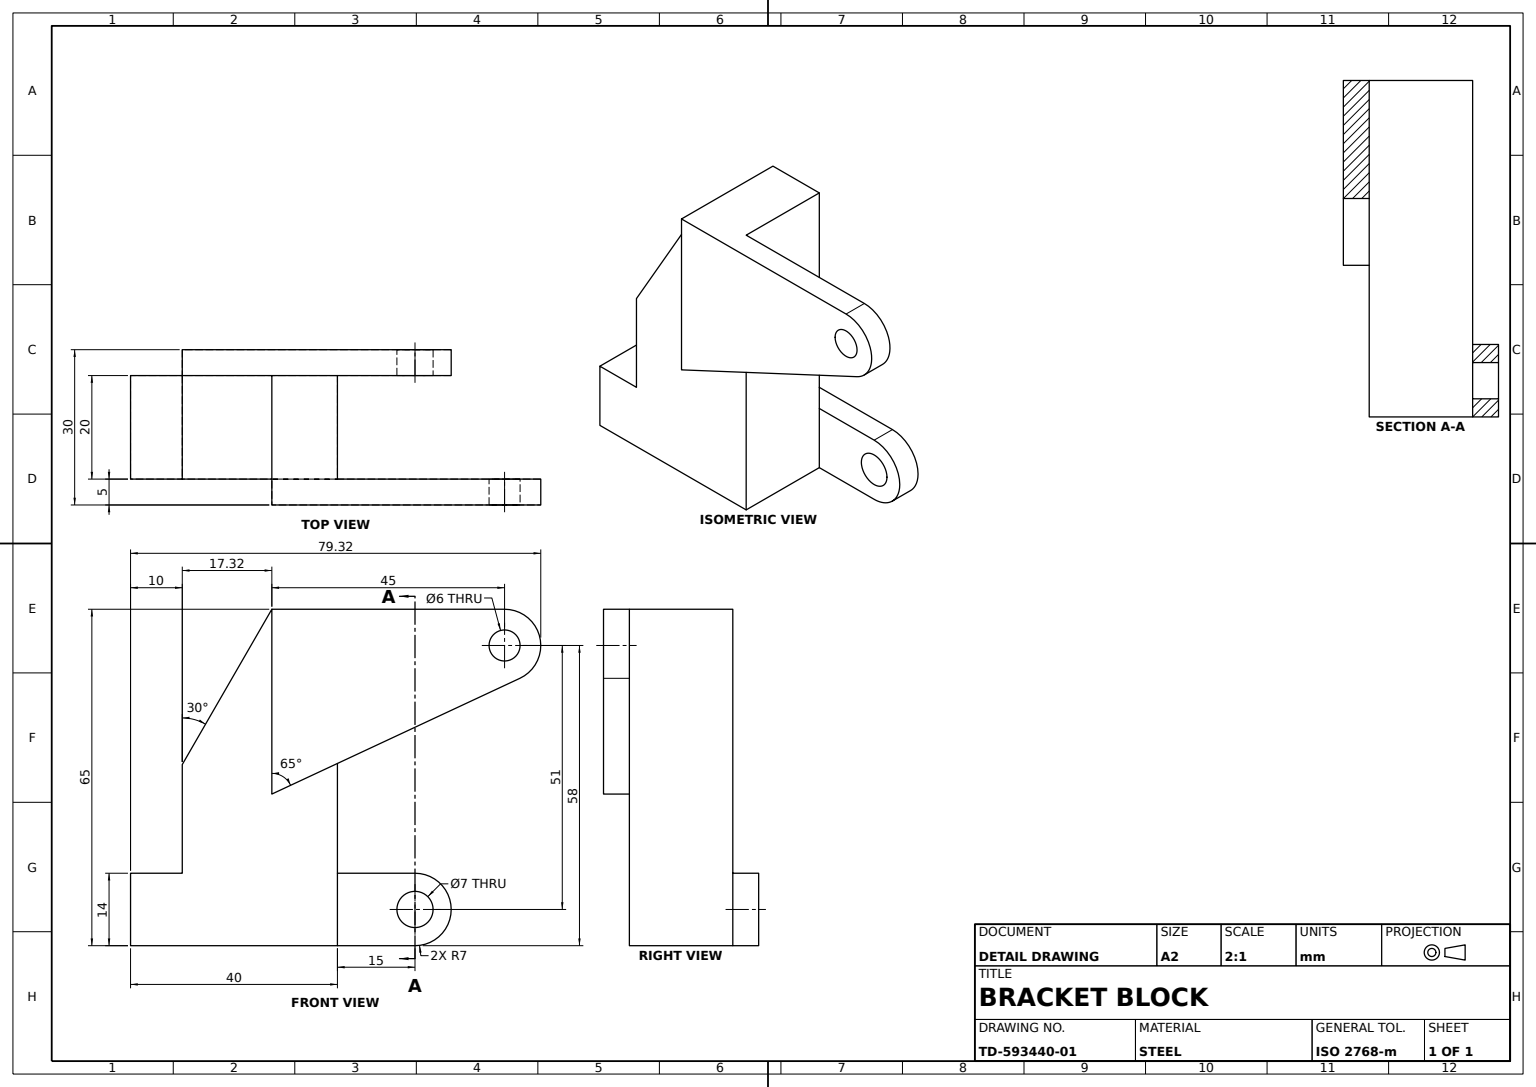
from build123d import *

# Parameters (mm, degrees)
BASE_BLOCK_SKETCH_W    = 40
BASE_BLOCK_SKETCH_H    = 20
BASE_BLOCK_DEPTH       = 14
UPRIGHT_SKETCH_W       = 30
UPRIGHT_SKETCH_H       = 20
UPRIGHT_BLOCK_DEPTH    = 51
ANGLED_CUT_30DEG_DEPTH = 51
UPPER_LUG_SKETCH_R     = 3
UPPER_LUG_DEPTH        = 5
LOWER_LUG_SKETCH_R     = 3.5
LOWER_LUG_DEPTH        = 5


with BuildPart() as part:
    # Base Block Sketch → Base Block (new body)
    with BuildSketch(Plane(origin=(0, 0, 0), x_dir=(1, 0, 0), z_dir=(0, 1, 0))):
        with Locations((20, -10)):
            Rectangle(BASE_BLOCK_SKETCH_W, BASE_BLOCK_SKETCH_H)
    extrude(amount=BASE_BLOCK_DEPTH)

    # Upright Sketch → Upright Block (add)
    with BuildSketch(Plane(origin=(0, 14, 0), x_dir=(1, 0, 0), z_dir=(0, 1, 0))):
        with Locations((25, -10)):
            Rectangle(UPRIGHT_SKETCH_W, UPRIGHT_SKETCH_H)
    extrude(amount=UPRIGHT_BLOCK_DEPTH)

    # Angled Cut Sketch 30deg → Angled Cut 30deg (cut)
    with BuildSketch(Plane.XY.offset(20)):
        Polygon((10, 65), (10, 35), (27.320508076, 65), align=None)
    extrude(amount=-ANGLED_CUT_30DEG_DEPTH, mode=Mode.SUBTRACT)

    # Upper Lug Sketch → Upper Lug (add)
    with BuildSketch(Plane.XY.offset(20)):
        with BuildLine():
            Line((27.320508076, 65), (27.320508076, 29.29250995))
            Line((27.320508076, 29.29250995), (75.278835908, 51.655845491))
            ThreePointArc((75.278835908, 51.655845491), (79.154580126, 59.515077298), (72.320508076, 65))
            Line((72.320508076, 65), (27.320508076, 65))
        make_face()
        with Locations((72.320508076, 58)):
            Circle(UPPER_LUG_SKETCH_R, mode=Mode.SUBTRACT)
    extrude(amount=UPPER_LUG_DEPTH)

    # Lower Lug Sketch → Lower Lug (add)
    with BuildSketch(Plane(origin=(0, 0, 0), x_dir=(-1, 0, 0), z_dir=(0, 0, -1))):
        with BuildLine():
            Line((-10, 14), (-55, 14))
            ThreePointArc((-55, 14), (-62, 7), (-55, 0))
            Line((-55, 0), (-10, 0))
            Line((-10, 0), (-10, 14))
        make_face()
        with Locations((-55, 7)):
            Circle(LOWER_LUG_SKETCH_R, mode=Mode.SUBTRACT)
    extrude(amount=LOWER_LUG_DEPTH)


solid = part.part
